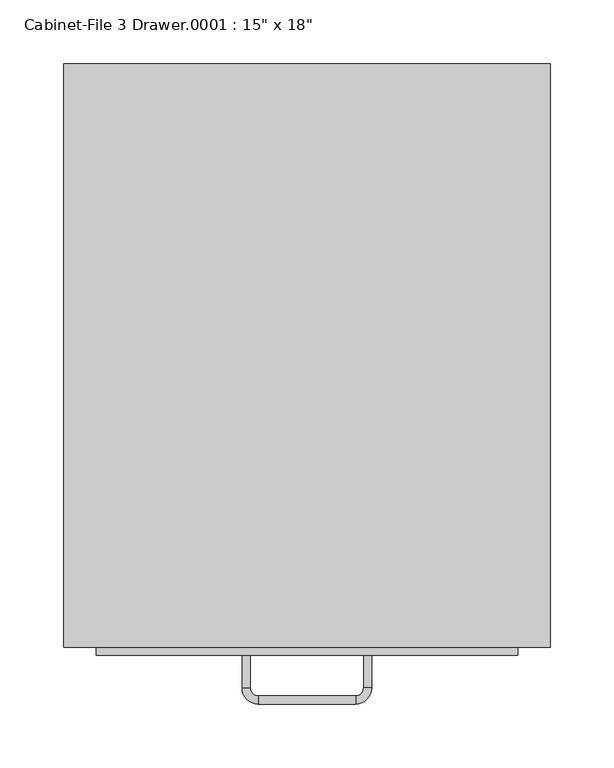
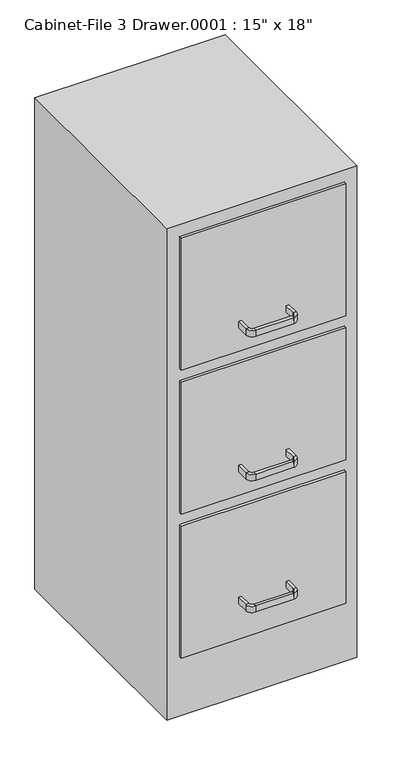
"""IFC4 building model written with IfcOpenShell, lengths in millimetres: furniture geometry."""

from ifc_helpers import new_model, si_unit, frame, origin, origin_with_axes, place, context, project, spatial, polyline, circle_curve, outline, extrude, source, transform, mapped, element, save
from ifc_brep_helpers import plane_surface, cylinder_surface, revolved_surface, advanced_brep


def furniture_552c1472(model_context):
    return source(origin(), model_context, "Body", "SolidModel", [
        extrude(outline(polyline([(62.603553, 86.4656999), (62.603553, -370.7343001), (-318.396447, -370.7343001), (-318.396447, 86.4656999), (62.603553, 86.4656999)])), origin_with_axes(), (0.0, 0.0, 1.0), 1041.4),
        extrude(outline(polyline([(37.203553, -377.0843001), (-292.996447, -377.0843001), (-292.996447, -370.7343001), (37.203553, -370.7343001), (37.203553, -377.0843001)])), frame((0.0, 0.0, 736.6), z_axis=(0.0, 0.0, 1.0), x_axis=(1.0, 0.0, 0.0)), (0.0, 0.0, 1.0), 279.4),
        extrude(outline(polyline([(37.203553, -377.0843001), (-292.996447, -377.0843001), (-292.996447, -370.7343001), (37.203553, -370.7343001), (37.203553, -377.0843001)])), frame((0.0, 0.0, 431.8), z_axis=(0.0, 0.0, 1.0), x_axis=(1.0, 0.0, 0.0)), (0.0, 0.0, 1.0), 279.4),
        extrude(outline(polyline([(37.203553, -377.0843001), (-292.996447, -377.0843001), (-292.996447, -370.7343001), (37.203553, -370.7343001), (37.203553, -377.0843001)])), frame((0.0, 0.0, 127.0), z_axis=(0.0, 0.0, 1.0), x_axis=(1.0, 0.0, 0.0)), (0.0, 0.0, 1.0), 279.4),
        advanced_brep(
        [(-172.346447, -377.0843001, 203.2), (-178.696447, -377.0843001, 203.2), (-178.696447, -377.0843001, 215.9), (-172.346447, -377.0843001, 215.9), (-172.346447, -402.4843001, 203.2), (-178.696447, -402.4843001, 203.2), (-178.696447, -402.4843001, 215.9), (-172.346447, -402.4843001, 215.9), (-165.996447, -415.1843001, 203.2), (-165.996447, -408.8343001, 203.2), (-165.996447, -415.1843001, 215.9), (-165.996447, -408.8343001, 215.9), (-89.796447, -408.8343001, 203.2), (-89.796447, -415.1843001, 203.2), (-89.796447, -415.1843001, 215.9), (-89.796447, -408.8343001, 215.9), (-77.096447, -402.4843001, 203.2), (-83.446447, -402.4843001, 203.2), (-77.096447, -402.4843001, 215.9), (-83.446447, -402.4843001, 215.9), (-83.446447, -377.0843001, 203.2), (-83.446447, -377.0843001, 215.9), (-77.096447, -377.0843001, 215.9), (-77.096447, -377.0843001, 203.2)],
        [
            (0, 1),
            (1, 2),
            (2, 3),
            (3, 0),
            (0, 4),
            (4, 5),
            (5, 1),
            (5, 6),
            (6, 2),
            (6, 7),
            (7, 3),
            (7, 4),
            (8, 5, circle_curve(frame((-165.996447, -402.4843001, 203.2), z_axis=(0.0, 0.0, -1.0), x_axis=(-1.0, 0.0, 0.0)), 12.7)),
            (4, 9, circle_curve(frame((-165.996447, -402.4843001, 203.2), z_axis=(0.0, 0.0, 1.0), x_axis=(-1.0, 0.0, 0.0)), 6.35)),
            (9, 8),
            (10, 6, circle_curve(frame((-165.996447, -402.4843001, 215.9), z_axis=(0.0, 0.0, -1.0), x_axis=(-1.0, 0.0, 0.0)), 12.7)),
            (8, 10),
            (11, 7, circle_curve(frame((-165.996447, -402.4843001, 215.9), z_axis=(0.0, 0.0, -1.0), x_axis=(-1.0, 0.0, 0.0)), 6.35)),
            (10, 11),
            (11, 9),
            (9, 12),
            (12, 13),
            (13, 8),
            (13, 14),
            (14, 10),
            (14, 15),
            (15, 11),
            (15, 12),
            (16, 13, circle_curve(frame((-89.796447, -402.4843001, 203.2), z_axis=(0.0, 0.0, -1.0), x_axis=(0.0, -1.0, 0.0)), 12.7)),
            (12, 17, circle_curve(frame((-89.796447, -402.4843001, 203.2), z_axis=(0.0, 0.0, 1.0), x_axis=(0.0, -1.0, 0.0)), 6.35)),
            (17, 16),
            (18, 14, circle_curve(frame((-89.796447, -402.4843001, 215.9), z_axis=(0.0, 0.0, -1.0), x_axis=(0.0, -1.0, 0.0)), 12.7)),
            (16, 18),
            (19, 15, circle_curve(frame((-89.796447, -402.4843001, 215.9), z_axis=(0.0, 0.0, -1.0), x_axis=(0.0, -1.0, 0.0)), 6.35)),
            (18, 19),
            (19, 17),
            (20, 21),
            (21, 22),
            (22, 23),
            (23, 20),
            (17, 20),
            (23, 16),
            (22, 18),
            (21, 19),
        ],
        [
            plane_surface(frame((-978.8216451, -377.0843001, 0.0), z_axis=(0.0, 1.0, 0.0), x_axis=(0.0, 0.0, -1.0))),
            plane_surface(frame((-172.346447, -377.0843001, 203.2), z_axis=(0.0, 0.0, -1.0), x_axis=(0.0, -1.0, 0.0))),
            plane_surface(frame((-178.696447, -377.0843001, 203.2), z_axis=(-1.0, 0.0, 0.0), x_axis=(0.0, -1.0, 0.0))),
            plane_surface(frame((-178.696447, -377.0843001, 215.9), z_axis=(0.0, 0.0, 1.0), x_axis=(0.0, -1.0, 0.0))),
            plane_surface(frame((-172.346447, -377.0843001, 215.9), z_axis=(1.0, 0.0, 0.0), x_axis=(0.0, -1.0, 0.0))),
            plane_surface(frame((-165.996447, -402.4843001, 203.2), z_axis=(0.0, 0.0, -1.0), x_axis=(-1.0, 0.0, 0.0))),
            cylinder_surface(frame((-165.996447, -402.4843001, 0.0), z_axis=(0.0, 0.0, 1.0), x_axis=(-1.0, 0.0, 0.0)), 12.7),
            plane_surface(frame((-165.996447, -402.4843001, 215.9), z_axis=(0.0, 0.0, 1.0), x_axis=(-1.0, 0.0, 0.0))),
            revolved_surface(polyline([(-172.34644699999998, -402.4843001, 215.9), (-172.34644699999998, -402.4843001, 203.2)]), (-165.996447, -402.4843001, 0.0), (0.0, 0.0, 1.0)),
            plane_surface(frame((-165.996447, -408.8343001, 203.2), z_axis=(0.0, 0.0, -1.0), x_axis=(1.0, 0.0, 0.0))),
            plane_surface(frame((-165.996447, -415.1843001, 203.2), z_axis=(0.0, -1.0, 0.0), x_axis=(1.0, 0.0, 0.0))),
            plane_surface(frame((-165.996447, -415.1843001, 215.9), z_axis=(0.0, 0.0, 1.0), x_axis=(1.0, 0.0, 0.0))),
            plane_surface(frame((-165.996447, -408.8343001, 215.9), z_axis=(0.0, 1.0, 0.0), x_axis=(1.0, 0.0, 0.0))),
            plane_surface(frame((-89.796447, -402.4843001, 203.2), z_axis=(0.0, 0.0, -1.0), x_axis=(0.0, -1.0, 0.0))),
            cylinder_surface(frame((-89.796447, -402.4843001, 0.0), z_axis=(0.0, 0.0, 1.0), x_axis=(0.0, -1.0, 0.0)), 12.7),
            plane_surface(frame((-89.796447, -402.4843001, 215.9), z_axis=(0.0, 0.0, 1.0), x_axis=(0.0, -1.0, 0.0))),
            revolved_surface(polyline([(-89.796447, -408.8343001, 215.9), (-89.796447, -408.8343001, 203.2)]), (-89.796447, -402.4843001, 0.0), (0.0, 0.0, 1.0)),
            plane_surface(frame((-877.2216451, -377.0843001, 0.0), z_axis=(0.0, 1.0, 0.0), x_axis=(0.0, 0.0, 1.0))),
            plane_surface(frame((-83.446447, -402.4843001, 203.2), z_axis=(0.0, 0.0, -1.0), x_axis=(0.0, 1.0, 0.0))),
            plane_surface(frame((-77.096447, -402.4843001, 203.2), z_axis=(1.0, 0.0, 0.0), x_axis=(0.0, 1.0, 0.0))),
            plane_surface(frame((-77.096447, -402.4843001, 215.9), z_axis=(0.0, 0.0, 1.0), x_axis=(0.0, 1.0, 0.0))),
            plane_surface(frame((-83.446447, -402.4843001, 215.9), z_axis=(-1.0, 0.0, 0.0), x_axis=(0.0, 1.0, 0.0))),
        ],
        [
            (0, [[1, 2, 3, 4]]),
            (1, [[-1, 5, 6, 7]]),
            (2, [[-2, -7, 8, 9]]),
            (3, [[-3, -9, 10, 11]]),
            (4, [[-4, -11, 12, -5]]),
            (5, [[13, -6, 14, 15]]),
            (6, [[16, -8, -13, 17]]),
            (7, [[18, -10, -16, 19]]),
            (8, [[-14, -12, -18, 20]]),
            (9, [[-15, 21, 22, 23]]),
            (10, [[-17, -23, 24, 25]]),
            (11, [[-19, -25, 26, 27]]),
            (12, [[-20, -27, 28, -21]]),
            (13, [[29, -22, 30, 31]]),
            (14, [[32, -24, -29, 33]]),
            (15, [[34, -26, -32, 35]]),
            (16, [[-30, -28, -34, 36]]),
            (17, [[37, 38, 39, 40]]),
            (18, [[-31, 41, -40, 42]]),
            (19, [[-33, -42, -39, 43]]),
            (20, [[-35, -43, -38, 44]]),
            (21, [[-36, -44, -37, -41]]),
        ],
    ),
        advanced_brep(
        [(-172.346447, -377.0843001, 482.6), (-178.696447, -377.0843001, 482.6), (-178.696447, -377.0843001, 495.3), (-172.346447, -377.0843001, 495.3), (-172.346447, -402.4843001, 482.6), (-178.696447, -402.4843001, 482.6), (-178.696447, -402.4843001, 495.3), (-172.346447, -402.4843001, 495.3), (-165.996447, -415.1843001, 482.6), (-165.996447, -408.8343001, 482.6), (-165.996447, -415.1843001, 495.3), (-165.996447, -408.8343001, 495.3), (-89.796447, -408.8343001, 482.6), (-89.796447, -415.1843001, 482.6), (-89.796447, -415.1843001, 495.3), (-89.796447, -408.8343001, 495.3), (-77.096447, -402.4843001, 482.6), (-83.446447, -402.4843001, 482.6), (-77.096447, -402.4843001, 495.3), (-83.446447, -402.4843001, 495.3), (-83.446447, -377.0843001, 482.6), (-83.446447, -377.0843001, 495.3), (-77.096447, -377.0843001, 495.3), (-77.096447, -377.0843001, 482.6)],
        [
            (0, 1),
            (1, 2),
            (2, 3),
            (3, 0),
            (0, 4),
            (4, 5),
            (5, 1),
            (5, 6),
            (6, 2),
            (6, 7),
            (7, 3),
            (7, 4),
            (8, 5, circle_curve(frame((-165.996447, -402.4843001, 482.6), z_axis=(0.0, 0.0, -1.0), x_axis=(-1.0, 0.0, 0.0)), 12.7)),
            (4, 9, circle_curve(frame((-165.996447, -402.4843001, 482.6), z_axis=(0.0, 0.0, 1.0), x_axis=(-1.0, 0.0, 0.0)), 6.35)),
            (9, 8),
            (10, 6, circle_curve(frame((-165.996447, -402.4843001, 495.3), z_axis=(0.0, 0.0, -1.0), x_axis=(-1.0, 0.0, 0.0)), 12.7)),
            (8, 10),
            (11, 7, circle_curve(frame((-165.996447, -402.4843001, 495.3), z_axis=(0.0, 0.0, -1.0), x_axis=(-1.0, 0.0, 0.0)), 6.35)),
            (10, 11),
            (11, 9),
            (9, 12),
            (12, 13),
            (13, 8),
            (13, 14),
            (14, 10),
            (14, 15),
            (15, 11),
            (15, 12),
            (16, 13, circle_curve(frame((-89.796447, -402.4843001, 482.6), z_axis=(0.0, 0.0, -1.0), x_axis=(0.0, -1.0, 0.0)), 12.7)),
            (12, 17, circle_curve(frame((-89.796447, -402.4843001, 482.6), z_axis=(0.0, 0.0, 1.0), x_axis=(0.0, -1.0, 0.0)), 6.35)),
            (17, 16),
            (18, 14, circle_curve(frame((-89.796447, -402.4843001, 495.3), z_axis=(0.0, 0.0, -1.0), x_axis=(0.0, -1.0, 0.0)), 12.7)),
            (16, 18),
            (19, 15, circle_curve(frame((-89.796447, -402.4843001, 495.3), z_axis=(0.0, 0.0, -1.0), x_axis=(0.0, -1.0, 0.0)), 6.35)),
            (18, 19),
            (19, 17),
            (20, 21),
            (21, 22),
            (22, 23),
            (23, 20),
            (17, 20),
            (23, 16),
            (22, 18),
            (21, 19),
        ],
        [
            plane_surface(frame((-978.8216451, -377.0843001, 0.0), z_axis=(0.0, 1.0, 0.0), x_axis=(0.0, 0.0, -1.0))),
            plane_surface(frame((-172.346447, -377.0843001, 482.6), z_axis=(0.0, 0.0, -1.0), x_axis=(0.0, -1.0, 0.0))),
            plane_surface(frame((-178.696447, -377.0843001, 482.6), z_axis=(-1.0, 0.0, 0.0), x_axis=(0.0, -1.0, 0.0))),
            plane_surface(frame((-178.696447, -377.0843001, 495.3), z_axis=(0.0, 0.0, 1.0), x_axis=(0.0, -1.0, 0.0))),
            plane_surface(frame((-172.346447, -377.0843001, 495.3), z_axis=(1.0, 0.0, 0.0), x_axis=(0.0, -1.0, 0.0))),
            plane_surface(frame((-165.996447, -402.4843001, 482.6), z_axis=(0.0, 0.0, -1.0), x_axis=(-1.0, 0.0, 0.0))),
            cylinder_surface(frame((-165.996447, -402.4843001, 0.0), z_axis=(0.0, 0.0, 1.0), x_axis=(-1.0, 0.0, 0.0)), 12.7),
            plane_surface(frame((-165.996447, -402.4843001, 495.3), z_axis=(0.0, 0.0, 1.0), x_axis=(-1.0, 0.0, 0.0))),
            revolved_surface(polyline([(-172.34644699999998, -402.4843001, 495.3), (-172.34644699999998, -402.4843001, 482.6)]), (-165.996447, -402.4843001, 0.0), (0.0, 0.0, 1.0)),
            plane_surface(frame((-165.996447, -408.8343001, 482.6), z_axis=(0.0, 0.0, -1.0), x_axis=(1.0, 0.0, 0.0))),
            plane_surface(frame((-165.996447, -415.1843001, 482.6), z_axis=(0.0, -1.0, 0.0), x_axis=(1.0, 0.0, 0.0))),
            plane_surface(frame((-165.996447, -415.1843001, 495.3), z_axis=(0.0, 0.0, 1.0), x_axis=(1.0, 0.0, 0.0))),
            plane_surface(frame((-165.996447, -408.8343001, 495.3), z_axis=(0.0, 1.0, 0.0), x_axis=(1.0, 0.0, 0.0))),
            plane_surface(frame((-89.796447, -402.4843001, 482.6), z_axis=(0.0, 0.0, -1.0), x_axis=(0.0, -1.0, 0.0))),
            cylinder_surface(frame((-89.796447, -402.4843001, 0.0), z_axis=(0.0, 0.0, 1.0), x_axis=(0.0, -1.0, 0.0)), 12.7),
            plane_surface(frame((-89.796447, -402.4843001, 495.3), z_axis=(0.0, 0.0, 1.0), x_axis=(0.0, -1.0, 0.0))),
            revolved_surface(polyline([(-89.796447, -408.8343001, 495.3), (-89.796447, -408.8343001, 482.6)]), (-89.796447, -402.4843001, 0.0), (0.0, 0.0, 1.0)),
            plane_surface(frame((-877.2216451, -377.0843001, 0.0), z_axis=(0.0, 1.0, 0.0), x_axis=(0.0, 0.0, 1.0))),
            plane_surface(frame((-83.446447, -402.4843001, 482.6), z_axis=(0.0, 0.0, -1.0), x_axis=(0.0, 1.0, 0.0))),
            plane_surface(frame((-77.096447, -402.4843001, 482.6), z_axis=(1.0, 0.0, 0.0), x_axis=(0.0, 1.0, 0.0))),
            plane_surface(frame((-77.096447, -402.4843001, 495.3), z_axis=(0.0, 0.0, 1.0), x_axis=(0.0, 1.0, 0.0))),
            plane_surface(frame((-83.446447, -402.4843001, 495.3), z_axis=(-1.0, 0.0, 0.0), x_axis=(0.0, 1.0, 0.0))),
        ],
        [
            (0, [[1, 2, 3, 4]]),
            (1, [[-1, 5, 6, 7]]),
            (2, [[-2, -7, 8, 9]]),
            (3, [[-3, -9, 10, 11]]),
            (4, [[-4, -11, 12, -5]]),
            (5, [[13, -6, 14, 15]]),
            (6, [[16, -8, -13, 17]]),
            (7, [[18, -10, -16, 19]]),
            (8, [[-14, -12, -18, 20]]),
            (9, [[-15, 21, 22, 23]]),
            (10, [[-17, -23, 24, 25]]),
            (11, [[-19, -25, 26, 27]]),
            (12, [[-20, -27, 28, -21]]),
            (13, [[29, -22, 30, 31]]),
            (14, [[32, -24, -29, 33]]),
            (15, [[34, -26, -32, 35]]),
            (16, [[-30, -28, -34, 36]]),
            (17, [[37, 38, 39, 40]]),
            (18, [[-31, 41, -40, 42]]),
            (19, [[-33, -42, -39, 43]]),
            (20, [[-35, -43, -38, 44]]),
            (21, [[-36, -44, -37, -41]]),
        ],
    ),
        advanced_brep(
        [(-172.346447, -377.0843001, 787.4), (-178.696447, -377.0843001, 787.4), (-178.696447, -377.0843001, 800.1), (-172.346447, -377.0843001, 800.1), (-172.346447, -402.4843001, 787.4), (-178.696447, -402.4843001, 787.4), (-178.696447, -402.4843001, 800.1), (-172.346447, -402.4843001, 800.1), (-165.996447, -415.1843001, 787.4), (-165.996447, -408.8343001, 787.4), (-165.996447, -415.1843001, 800.1), (-165.996447, -408.8343001, 800.1), (-89.796447, -408.8343001, 787.4), (-89.796447, -415.1843001, 787.4), (-89.796447, -415.1843001, 800.1), (-89.796447, -408.8343001, 800.1), (-77.096447, -402.4843001, 787.4), (-83.446447, -402.4843001, 787.4), (-77.096447, -402.4843001, 800.1), (-83.446447, -402.4843001, 800.1), (-83.446447, -377.0843001, 787.4), (-83.446447, -377.0843001, 800.1), (-77.096447, -377.0843001, 800.1), (-77.096447, -377.0843001, 787.4)],
        [
            (0, 1),
            (1, 2),
            (2, 3),
            (3, 0),
            (0, 4),
            (4, 5),
            (5, 1),
            (5, 6),
            (6, 2),
            (6, 7),
            (7, 3),
            (7, 4),
            (8, 5, circle_curve(frame((-165.996447, -402.4843001, 787.4), z_axis=(0.0, 0.0, -1.0), x_axis=(-1.0, 0.0, 0.0)), 12.7)),
            (4, 9, circle_curve(frame((-165.996447, -402.4843001, 787.4), z_axis=(0.0, 0.0, 1.0), x_axis=(-1.0, 0.0, 0.0)), 6.35)),
            (9, 8),
            (10, 6, circle_curve(frame((-165.996447, -402.4843001, 800.1), z_axis=(0.0, 0.0, -1.0), x_axis=(-1.0, 0.0, 0.0)), 12.7)),
            (8, 10),
            (11, 7, circle_curve(frame((-165.996447, -402.4843001, 800.1), z_axis=(0.0, 0.0, -1.0), x_axis=(-1.0, 0.0, 0.0)), 6.35)),
            (10, 11),
            (11, 9),
            (9, 12),
            (12, 13),
            (13, 8),
            (13, 14),
            (14, 10),
            (14, 15),
            (15, 11),
            (15, 12),
            (16, 13, circle_curve(frame((-89.796447, -402.4843001, 787.4), z_axis=(0.0, 0.0, -1.0), x_axis=(0.0, -1.0, 0.0)), 12.7)),
            (12, 17, circle_curve(frame((-89.796447, -402.4843001, 787.4), z_axis=(0.0, 0.0, 1.0), x_axis=(0.0, -1.0, 0.0)), 6.35)),
            (17, 16),
            (18, 14, circle_curve(frame((-89.796447, -402.4843001, 800.1), z_axis=(0.0, 0.0, -1.0), x_axis=(0.0, -1.0, 0.0)), 12.7)),
            (16, 18),
            (19, 15, circle_curve(frame((-89.796447, -402.4843001, 800.1), z_axis=(0.0, 0.0, -1.0), x_axis=(0.0, -1.0, 0.0)), 6.35)),
            (18, 19),
            (19, 17),
            (20, 21),
            (21, 22),
            (22, 23),
            (23, 20),
            (17, 20),
            (23, 16),
            (22, 18),
            (21, 19),
        ],
        [
            plane_surface(frame((-978.8216451, -377.0843001, 0.0), z_axis=(0.0, 1.0, 0.0), x_axis=(0.0, 0.0, -1.0))),
            plane_surface(frame((-172.346447, -377.0843001, 787.4), z_axis=(0.0, 0.0, -1.0), x_axis=(0.0, -1.0, 0.0))),
            plane_surface(frame((-178.696447, -377.0843001, 787.4), z_axis=(-1.0, 0.0, 0.0), x_axis=(0.0, -1.0, 0.0))),
            plane_surface(frame((-178.696447, -377.0843001, 800.1), z_axis=(0.0, 0.0, 1.0), x_axis=(0.0, -1.0, 0.0))),
            plane_surface(frame((-172.346447, -377.0843001, 800.1), z_axis=(1.0, 0.0, 0.0), x_axis=(0.0, -1.0, 0.0))),
            plane_surface(frame((-165.996447, -402.4843001, 787.4), z_axis=(0.0, 0.0, -1.0), x_axis=(-1.0, 0.0, 0.0))),
            cylinder_surface(frame((-165.996447, -402.4843001, 0.0), z_axis=(0.0, 0.0, 1.0), x_axis=(-1.0, 0.0, 0.0)), 12.7),
            plane_surface(frame((-165.996447, -402.4843001, 800.1), z_axis=(0.0, 0.0, 1.0), x_axis=(-1.0, 0.0, 0.0))),
            revolved_surface(polyline([(-172.34644699999998, -402.4843001, 800.1), (-172.34644699999998, -402.4843001, 787.4)]), (-165.996447, -402.4843001, 0.0), (0.0, 0.0, 1.0)),
            plane_surface(frame((-165.996447, -408.8343001, 787.4), z_axis=(0.0, 0.0, -1.0), x_axis=(1.0, 0.0, 0.0))),
            plane_surface(frame((-165.996447, -415.1843001, 787.4), z_axis=(0.0, -1.0, 0.0), x_axis=(1.0, 0.0, 0.0))),
            plane_surface(frame((-165.996447, -415.1843001, 800.1), z_axis=(0.0, 0.0, 1.0), x_axis=(1.0, 0.0, 0.0))),
            plane_surface(frame((-165.996447, -408.8343001, 800.1), z_axis=(0.0, 1.0, 0.0), x_axis=(1.0, 0.0, 0.0))),
            plane_surface(frame((-89.796447, -402.4843001, 787.4), z_axis=(0.0, 0.0, -1.0), x_axis=(0.0, -1.0, 0.0))),
            cylinder_surface(frame((-89.796447, -402.4843001, 0.0), z_axis=(0.0, 0.0, 1.0), x_axis=(0.0, -1.0, 0.0)), 12.7),
            plane_surface(frame((-89.796447, -402.4843001, 800.1), z_axis=(0.0, 0.0, 1.0), x_axis=(0.0, -1.0, 0.0))),
            revolved_surface(polyline([(-89.796447, -408.8343001, 800.1), (-89.796447, -408.8343001, 787.4)]), (-89.796447, -402.4843001, 0.0), (0.0, 0.0, 1.0)),
            plane_surface(frame((-877.2216451, -377.0843001, 0.0), z_axis=(0.0, 1.0, 0.0), x_axis=(0.0, 0.0, 1.0))),
            plane_surface(frame((-83.446447, -402.4843001, 787.4), z_axis=(0.0, 0.0, -1.0), x_axis=(0.0, 1.0, 0.0))),
            plane_surface(frame((-77.096447, -402.4843001, 787.4), z_axis=(1.0, 0.0, 0.0), x_axis=(0.0, 1.0, 0.0))),
            plane_surface(frame((-77.096447, -402.4843001, 800.1), z_axis=(0.0, 0.0, 1.0), x_axis=(0.0, 1.0, 0.0))),
            plane_surface(frame((-83.446447, -402.4843001, 800.1), z_axis=(-1.0, 0.0, 0.0), x_axis=(0.0, 1.0, 0.0))),
        ],
        [
            (0, [[1, 2, 3, 4]]),
            (1, [[-1, 5, 6, 7]]),
            (2, [[-2, -7, 8, 9]]),
            (3, [[-3, -9, 10, 11]]),
            (4, [[-4, -11, 12, -5]]),
            (5, [[13, -6, 14, 15]]),
            (6, [[16, -8, -13, 17]]),
            (7, [[18, -10, -16, 19]]),
            (8, [[-14, -12, -18, 20]]),
            (9, [[-15, 21, 22, 23]]),
            (10, [[-17, -23, 24, 25]]),
            (11, [[-19, -25, 26, 27]]),
            (12, [[-20, -27, 28, -21]]),
            (13, [[29, -22, 30, 31]]),
            (14, [[32, -24, -29, 33]]),
            (15, [[34, -26, -32, 35]]),
            (16, [[-30, -28, -34, 36]]),
            (17, [[37, 38, 39, 40]]),
            (18, [[-31, 41, -40, 42]]),
            (19, [[-33, -42, -39, 43]]),
            (20, [[-35, -43, -38, 44]]),
            (21, [[-36, -44, -37, -41]]),
        ],
    ),
    ])


if __name__ == "__main__":
    model = new_model("IFC4")
    model_context = context("Model", 3, world=origin())
    ifc_project = project(units=[si_unit("LENGTHUNIT", "METRE", prefix="MILLI")], contexts=[model_context])
    site = spatial("IfcSite", under=ifc_project)
    building = spatial("IfcBuilding", under=site)
    placement = place(None, origin())
    furniture_shape = furniture_552c1472(model_context)
    element("IfcFurniture", 1, ObjectType="Cabinet-File 3 Drawer.0001 : 15\" x 18\"", at=placement, inside=building, context=model_context, shape_type="MappedRepresentation", body=[
        mapped(furniture_shape, transform((0.0, 0.0, 0.0), x_axis=(1.0, 0.0, 0.0), y_axis=(0.0, 1.0, 0.0), z_axis=(0.0, 0.0, 1.0))),
    ])
    save(model, "model.ifc")

# Revit data of these elements
# Type "Cabinet-File 3 Drawer.0001 : 15\" x 18\""
#   Assembly Code = "E2020200"
#   Depth = 1' - 6"
#   Height = 3' - 5"
#   Width = 1' - 3"
#   Cabinet Material = Steel, Paint Finish, Ivory, Glossy
#   Handle Material = Steel, Chrome Plated
#   Default Elevation = 0
# Element 1 (IfcFurniture, "Cabinet-File 3 Drawer.0001 : 15\" x 18\"")
#   Materials on its faces: "Steel, Chrome Plated", "Steel, Paint Finish, Ivory, Glossy"
# Materials
#   "Steel, Paint Finish, Ivory, Glossy": class "Metal", colour RGB 247 247 239, transparency 0, Description = "Steel, paint finish, ivory, glossy", Cost = 0
#   "Steel, Chrome Plated": class "Metal", colour RGB 17 17 17, transparency 0, Description = "Chromiuim plated steel", Cost = 0
